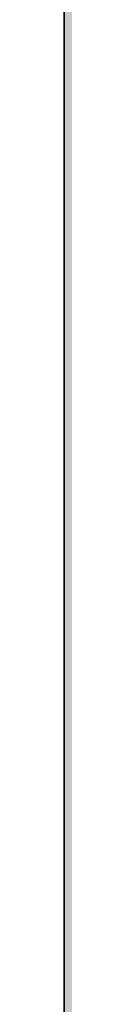
# Model space of a CAD drawing. Units: inches. Extents: x 2091 to 2899, y 967 to 2217.
# Tile 77 of 256: x 2203 to 2203, y 1114 to 1131. Entities that reach past the tile are written whole.
import ezdxf

# ---------------------------------------------------------------- set-up
doc = ezdxf.new("R2010")
doc.units = ezdxf.units.IN
doc.layers.add('A-WALL-PATT', color=141, linetype='Continuous', lineweight=13, true_color=0xadddf7)
doc.layers.add('C-PROP', color=7, linetype='Continuous', lineweight=35)

msp = doc.modelspace()

# ---------------------------------------------------------------- hatches: boundary and pattern name
at = {"layer": 'A-WALL-PATT'}
h = msp.add_hatch(color=256, dxfattribs=at)
h.dxf.hatch_style = 1
h.paths.add_polyline_path([(2212.144, 1941.419), (2387.644, 1941.419), (2387.644, 1824.419), (2392.144, 1824.419), (2392.144, 1941.419), (2609.644, 1941.419), (2609.644, 1825.919), (2614.144, 1825.919), (2614.144, 1941.419), (2794.144, 1941.419), (2794.144, 1928.762), (2803.144, 1928.762), (2803.144, 2050.919), (2203.144, 2050.919), (2203.144, 1900.758), (2212.144, 1900.758)])
h.paths.add_polyline_path([(2212.144, 1945.919), (2212.144, 2041.919), (2794.144, 2041.919), (2794.144, 1945.919), (2402.248, 1945.919), (2401.102, 1945.776), (2398.702, 1945.776)], flags=16)
h.paths.add_polyline_path([(2230.23, 1948.063), (2227.35, 1949.503), (2225.91, 1951.903), (2223.99, 1952.863), (2223.03, 1955.263), (2222.07, 1959.583), (2222.07, 1963.423), (2223.03, 1965.663), (2223.99, 1965.343), (2225.586, 1963.861), (2226.912, 1964.957), (2226.949, 1965.939), (2227.778, 1966.952), (2228.2, 1968.879), (2230.71, 1964.863), (2233.59, 1966.303), (2233.607, 1966.332), (2233.773, 1964.938), (2234.634, 1963.676), (2235.03, 1963.903), (2236.282, 1965.572), (2235.99, 1962.943), (2237.955, 1957.54), (2238.39, 1957.903), (2239.216, 1960.306), (2238.655, 1966.385), (2238.693, 1966.438), (2238.841, 1967.5), (2238.78, 1967.687), (2238.881, 1967.787), (2238.667, 1966.252), (2239.216, 1960.306), (2238.39, 1957.903), (2236.95, 1956.703), (2234.55, 1949.983)], flags=0)
h.paths.add_polyline_path([(2278.012, 1948.063), (2276.496, 1947.873), (2275.85, 1947.689), (2274.652, 1947.103)], flags=0)
h.paths.add_polyline_path([(2269.852, 1955.743), (2268.276, 1956.629), (2270.867, 1956.348), (2269.372, 1958.143), (2268.715, 1959.192), (2270.57, 1958.729), (2268.581, 1961.906), (2270.812, 1960.892), (2270.812, 1963.423), (2271.393, 1964.779), (2270.292, 1966.156), (2271.772, 1965.663), (2272.141, 1966.525), (2273.93, 1965.929), (2275.63, 1968.054), (2276.332, 1966.722), (2276.52, 1966.952), (2276.942, 1968.879), (2277.734, 1967.611), (2278.14, 1969.465), (2279.659, 1967.034), (2280.412, 1966.783), (2280.949, 1967.589), (2281.61, 1967.369), (2282.133, 1968.154), (2282.349, 1966.333), (2282.35, 1966.333), (2283.408, 1968.095), (2283.713, 1965.524), (2284.32, 1964.634), (2284.512, 1964.889), (2284.235, 1965.705), (2284.5, 1967.319), (2284.908, 1965.417), (2285.396, 1966.069), (2285.433, 1966.291), (2285.473, 1966.171), (2286.354, 1967.345), (2286.222, 1966.158), (2287.663, 1968.08), (2287.714, 1968.443), (2288.482, 1969.017), (2288.574, 1968.729), (2288.917, 1969.069), (2288.607, 1966.838), (2288.929, 1963.351), (2288.935, 1963.357), (2288.93, 1963.34), (2289.015, 1962.414), (2290.111, 1963.875), (2290.133, 1963.943), (2290.218, 1964.017), (2290.111, 1963.875), (2289.156, 1960.892), (2288.594, 1959.257), (2288.572, 1959.103), (2289.532, 1960.543), (2290.012, 1962.463), (2290.192, 1962.643), (2289.77, 1959.689), (2286.89, 1957.289), (2284.49, 1950.569), (2283.315, 1950.046), (2283.292, 1949.983), (2280.29, 1948.649), (2281.13, 1948.649), (2282.57, 1948.169), (2283.205, 1948.063), (2278.972, 1948.063), (2276.092, 1949.503), (2274.652, 1951.903), (2272.732, 1952.863)], flags=0)
h.paths.add_polyline_path([(2271.159, 1958.022), (2272.97, 1955.849), (2272.01, 1960.169), (2272.01, 1964.009), (2272.624, 1965.443), (2274.328, 1963.861), (2275.654, 1964.957), (2275.638, 1964.539), (2277.412, 1966.007), (2277.033, 1965.157), (2276.83, 1964.976), (2276.766, 1963.295), (2277.45, 1962.66), (2279.452, 1964.863), (2282.332, 1966.303), (2283.53, 1966.889), (2283.295, 1966.771), (2283.913, 1963.885), (2284.899, 1964.448), (2284.732, 1962.943), (2286.697, 1957.54), (2287.132, 1957.903), (2287.542, 1959.095), (2287.779, 1958.442), (2285.683, 1956.695), (2285.877, 1959.795), (2284.732, 1962.943), (2284.899, 1964.448), (2283.913, 1963.885), (2284.224, 1962.434), (2283.424, 1963.605), (2281.61, 1962.569), (2281.13, 1960.169), (2282.09, 1956.329), (2283.05, 1952.969), (2282.57, 1950.569), (2280.17, 1948.649), (2279.883, 1948.792), (2278.972, 1948.063), (2278.972, 1949.023), (2278.672, 1949.397), (2277.29, 1950.089), (2275.85, 1952.489), (2273.93, 1953.449), (2272.49, 1954.889), (2271.922, 1954.889), (2271.772, 1955.263)], flags=0)
h.paths.add_polyline_path([(2311.994, 1955.743), (2312.063, 1955.674), (2312.055, 1955.709)], flags=0)
h.paths.add_polyline_path([(2331.956, 1963.952), (2333.396, 1965.392), (2331.077, 1963.357), (2330.999, 1963.112)], flags=0)
h.paths.add_polyline_path([(2310.554, 1954.303), (2307.04, 1956.28), (2310.763, 1955.876), (2312.474, 1953.823), (2313.434, 1951.423), (2315.354, 1950.463), (2316.794, 1948.063), (2317.466, 1947.727), (2319.369, 1947.965), (2317.754, 1949.983), (2317.57, 1950.61), (2316.794, 1951.903), (2314.874, 1952.863), (2313.914, 1955.263), (2311.514, 1958.143), (2309.375, 1961.559), (2311.514, 1960.337), (2311.514, 1961.983), (2310.605, 1963.12), (2311.727, 1962.479), (2312.418, 1964.093), (2312.256, 1964.296), (2313.194, 1963.983), (2313.914, 1965.663), (2314.647, 1965.419), (2315.354, 1966.303), (2316.794, 1967.743), (2316.157, 1966.947), (2317.034, 1965.282), (2317.223, 1965.512), (2317.777, 1968.046), (2318.474, 1966.722), (2318.663, 1966.952), (2319.084, 1968.879), (2321.207, 1965.482), (2322.161, 1966.914), (2322.554, 1966.783), (2322.786, 1967.131), (2322.882, 1966.324), (2323.312, 1965.722), (2323.651, 1965.891), (2324.396, 1967.133), (2324.657, 1964.938), (2324.972, 1964.477), (2325.387, 1967.001), (2325.941, 1964.418), (2327.229, 1966.136), (2327.166, 1965.572), (2328.059, 1966.763), (2328.225, 1966.247), (2329.668, 1967.677), (2329.665, 1967.687), (2329.765, 1967.787), (2329.551, 1966.252), (2330.1, 1960.306), (2329.333, 1958.073), (2329.313, 1957.935), (2329.634, 1958.203), (2330.234, 1959.103), (2330.714, 1961.023), (2331.034, 1961.343), (2330.714, 1959.103), (2329.634, 1958.203), (2329.274, 1957.663), (2327.712, 1956.361), (2325.434, 1949.983), (2324.334, 1949.494), (2323.994, 1948.543), (2319.674, 1946.623), (2316.794, 1948.063), (2315.354, 1950.463), (2313.434, 1951.423)], flags=0)
h.paths.add_polyline_path([(2321.336, 1947.952), (2321.114, 1948.063), (2321.114, 1949.023), (2319.194, 1951.423), (2316.794, 1959.583), (2316.663, 1959.583), (2315.354, 1958.143), (2314.394, 1958.143), (2313.148, 1958.709), (2312.954, 1959.583), (2312.954, 1960.892), (2315.834, 1959.583), (2316.663, 1959.583), (2317.315, 1960.299), (2315.03, 1962.421), (2316.356, 1963.517), (2316.372, 1963.952), (2316.47, 1963.861), (2317.796, 1964.957), (2317.755, 1963.89), (2319.175, 1965.157), (2319.498, 1965.881), (2321.114, 1965.343), (2323.236, 1962.372), (2325.686, 1963.773), (2325.543, 1962.481), (2325.199, 1963.494), (2324.479, 1963.082), (2324.926, 1960.994), (2324.078, 1962.236), (2322.415, 1961.286), (2322.074, 1959.583), (2323.034, 1955.743), (2323.994, 1952.383), (2323.514, 1949.983), (2322.143, 1948.886), (2322.074, 1948.543)], flags=0)
h.paths.add_polyline_path([(2320.207, 1963.337), (2320.154, 1963.423), (2320.394, 1963.543)], flags=0)
h.paths.add_polyline_path([(2353.851, 1965.811), (2354.031, 1965.751), (2354.331, 1966.451), (2354.331, 1966.931)], flags=0)
h.paths.add_polyline_path([(2359.021, 1969.026), (2359.098, 1968.902), (2359.234, 1969.52), (2359.234, 1970)], flags=0)
h.paths.add_polyline_path([(2358.257, 1966.682), (2357.984, 1966.348), (2358.211, 1966.146), (2358.41, 1966.39)], flags=0)
h.paths.add_polyline_path([(2357.768, 1966.059), (2357.732, 1965.105), (2357.751, 1965.121), (2357.77, 1965.607), (2357.77, 1966.058)], flags=0)
h.paths.add_polyline_path([(2359.112, 1965.305), (2359.112, 1964.825), (2359.845, 1966.468), (2359.845, 1966.948)], flags=0)
h.paths.add_polyline_path([(2360.224, 1966.621), (2360.699, 1969.363), (2360.699, 1969.843), (2360.211, 1967.026), (2360.211, 1966.643)], flags=0)
h.paths.add_polyline_path([(2363.451, 1967.891), (2363.451, 1968.371), (2362.491, 1966.931), (2362.656, 1966.699)], flags=0)
h.paths.add_polyline_path([(2364.476, 1966.079), (2365.851, 1968.371), (2365.851, 1968.851), (2364.428, 1966.48)], flags=0)
h.paths.add_polyline_path([(2366.314, 1965.853), (2366.367, 1965.696), (2366.803, 1968.346), (2366.803, 1968.826)], flags=0)
h.paths.add_polyline_path([(2367.165, 1965.804), (2367.291, 1966.931), (2367.291, 1967.411), (2367.103, 1965.72)], flags=0)
h.paths.add_polyline_path([(2370.037, 1959.974), (2371.014, 1963.025), (2371.014, 1963.505), (2370.037, 1960.454)], flags=0)
h.paths.add_polyline_path([(2371.611, 1960.211), (2372.571, 1961.651), (2372.571, 1962.131), (2371.803, 1960.979)], flags=0)
h.paths.add_polyline_path([(2350.874, 1956.005), (2351.931, 1955.891), (2354.491, 1953.331), (2353.851, 1954.931), (2351.451, 1957.811), (2347.936, 1963.426), (2347.936, 1963.906), (2351.451, 1958.291), (2353.705, 1955.585), (2352.891, 1959.251), (2352.891, 1959.731), (2352.891, 1961.925), (2356.731, 1959.731), (2358.454, 1961.627), (2354.811, 1965.011), (2355.031, 1965.286), (2358.691, 1961.887), (2361.531, 1965.011), (2364.376, 1966.433), (2364.524, 1965.187), (2365.454, 1963.824), (2365.881, 1964.068), (2365.371, 1966.451), (2365.371, 1966.931), (2366.811, 1960.211), (2366.811, 1959.731), (2366.389, 1952.981), (2367.771, 1956.851), (2368.641, 1957.576), (2366.811, 1962.611), (2366.811, 1963.091), (2368.775, 1957.688), (2369.211, 1958.051), (2370.002, 1960.352), (2369.475, 1966.053), (2369.513, 1966.106), (2369.514, 1966.111), (2369.475, 1966.533), (2369.513, 1966.586), (2369.615, 1967.313), (2369.183, 1968.659), (2369.183, 1969.139), (2369.601, 1967.835), (2369.701, 1967.934), (2369.718, 1968.055), (2370.145, 1968.374), (2369.779, 1968.011), (2369.701, 1967.454), (2370.468, 1968.214), (2369.675, 1967.266), (2369.514, 1966.111), (2370.037, 1960.454), (2370.037, 1959.974), (2369.442, 1958.243), (2370.651, 1959.251), (2371.046, 1962.018), (2371.131, 1962.131), (2370.651, 1958.771), (2367.771, 1956.371), (2365.371, 1949.651), (2362.079, 1948.188), (2363.451, 1947.731), (2361.051, 1947.731), (2360.091, 1947.731), (2357.104, 1947.357), (2360.091, 1948.211), (2358.171, 1949.171), (2356.731, 1951.571), (2354.811, 1952.531), (2351.931, 1955.411)], flags=0)
h.paths.add_polyline_path([(2361.051, 1948.691), (2359.131, 1951.091), (2356.731, 1959.251), (2355.771, 1959.251), (2352.891, 1960.56), (2352.891, 1961.445), (2355.891, 1959.731), (2356.731, 1959.731), (2356.837, 1959.368), (2361.531, 1964.531), (2363.248, 1965.389), (2364.925, 1963.042), (2362.491, 1961.651), (2362.064, 1959.517), (2362.971, 1955.891), (2363.931, 1952.531), (2363.931, 1952.051), (2363.451, 1949.651), (2361.051, 1947.731)], flags=0)
h.paths.add_polyline_path([(2359.131, 1951.571), (2359.291, 1951.371), (2361.051, 1954.451), (2361.051, 1954.931)], flags=0)
h.paths.add_polyline_path([(2357.22, 1966.546), (2356.793, 1968.815), (2356.793, 1969.295), (2357.22, 1967.026)], flags=0)
h.paths.add_polyline_path([(2361.051, 1954.451), (2361.531, 1958.771), (2361.531, 1959.251), (2361.051, 1954.931)], flags=0)
h.paths.add_polyline_path([(2402.548, 1948.486), (2402.302, 1948.416), (2402.59, 1948.416)], flags=0)
h.paths.add_polyline_path([(2394.142, 1956.096), (2395.685, 1954.553), (2396.72, 1953.971), (2396.062, 1955.616), (2395.241, 1956.601), (2395.879, 1956.442), (2395.102, 1959.936), (2395.102, 1963.776), (2396.062, 1966.016), (2397.022, 1965.696), (2398.618, 1964.214), (2399.944, 1965.31), (2399.981, 1966.292), (2400.811, 1967.305), (2401.232, 1969.232), (2403.538, 1965.543), (2403.942, 1967.389), (2404.702, 1967.136), (2405.46, 1966.075), (2406.622, 1966.656), (2406.64, 1966.685), (2406.805, 1965.291), (2406.926, 1965.115), (2407.342, 1964.976), (2407.874, 1965.774), (2408.169, 1964.398), (2409.315, 1965.925), (2409.217, 1965.051), (2409.445, 1963.131), (2410.306, 1961.87), (2410.702, 1962.096), (2411.442, 1963.082), (2411.165, 1963.898), (2411.616, 1966.64), (2411.725, 1966.791), (2411.873, 1967.853), (2411.813, 1968.041), (2411.913, 1968.14), (2411.699, 1966.605), (2412.248, 1960.659), (2413.225, 1963.71), (2414.378, 1964.721), (2414.513, 1965.693), (2414.453, 1965.881), (2414.553, 1965.98), (2414.378, 1964.721), (2414.52, 1964.846), (2414.365, 1964.631), (2414.339, 1964.445), (2414.888, 1958.499), (2414.062, 1956.096), (2412.622, 1954.896), (2410.171, 1948.033), (2410.017, 1948.084), (2405.902, 1946.256), (2405.902, 1947.216), (2405.204, 1948.089), (2404.222, 1948.416), (2403.262, 1948.416), (2400.382, 1949.856), (2399.662, 1951.056), (2397.982, 1952.736), (2397.022, 1953.216), (2395.685, 1954.553), (2392.657, 1956.257)], flags=0)
h.paths.add_polyline_path([(2409.086, 1964.407), (2409.13, 1964.276), (2409.262, 1964.496)], flags=0)
h.paths.add_polyline_path([(2397.742, 1961.616), (2398.702, 1963.856), (2399.662, 1963.536), (2401.427, 1965.741), (2401.791, 1966.559), (2402.071, 1965.071), (2402.836, 1964.393), (2403.262, 1964.915), (2403.338, 1964.771), (2402.616, 1963.976), (2402.499, 1960.902), (2403.543, 1959.932), (2404.413, 1960.89), (2404.702, 1962.336), (2407.916, 1964.172), (2409.52, 1961.927), (2410.987, 1957.893), (2411.422, 1958.256), (2412.048, 1960.076), (2412.41, 1959.079), (2411.676, 1958.467), (2411.662, 1958.256), (2411.626, 1958.426), (2409.982, 1957.056), (2407.582, 1950.336), (2403.262, 1948.416), (2403.262, 1949.376), (2401.342, 1951.776), (2399.417, 1958.324), (2397.742, 1959.085), (2397.742, 1959.97), (2397.102, 1960.336), (2397.742, 1960.045)], flags=0)
h.paths.add_polyline_path([(2405.902, 1952.976), (2405.95, 1953.408), (2406.017, 1953.176)], flags=0)
h.paths.add_polyline_path([(2449.818, 1967.114), (2449.752, 1967.136), (2449.794, 1967.078)], flags=0)
h.paths.add_polyline_path([(2451.698, 1966.618), (2451.741, 1966.69), (2451.692, 1966.666)], flags=0)
h.paths.add_polyline_path([(2454.344, 1965.738), (2455.752, 1967.616), (2455.992, 1968.096), (2454.364, 1965.925)], flags=0)
h.paths.add_polyline_path([(2457.547, 1968.864), (2457.787, 1969.344), (2457.054, 1968.796), (2457.008, 1968.46)], flags=0)
h.paths.add_polyline_path([(2456.922, 1967.857), (2456.802, 1968.229), (2456.723, 1967.66)], flags=0)
h.paths.add_polyline_path([(2457.302, 1967.377), (2457.542, 1967.857), (2456.81, 1966.84), (2456.741, 1966.7), (2456.749, 1966.608)], flags=0)
h.paths.add_polyline_path([(2458.275, 1963.71), (2458.155, 1963.335), (2460.354, 1965.265), (2460.594, 1965.745)], flags=0)
h.paths.add_polyline_path([(2458.392, 1962.816), (2458.364, 1962.618), (2459.592, 1964.256), (2459.832, 1964.736)], flags=0)
h.paths.add_polyline_path([(2459.352, 1962.816), (2459.272, 1962.496), (2460.072, 1963.296), (2460.312, 1963.776)], flags=0)
h.paths.add_polyline_path([(2458.68, 1960.608), (2458.632, 1960.416), (2459.592, 1961.856), (2459.832, 1962.336)], flags=0)
h.paths.add_polyline_path([(2437.838, 1956.243), (2439.192, 1956.096), (2441.352, 1953.936), (2440.872, 1955.136), (2438.472, 1958.016), (2438.072, 1958.656), (2438.712, 1958.496), (2440.64, 1956.183), (2439.912, 1959.456), (2439.912, 1963.296), (2441.352, 1966.656), (2441.592, 1967.136), (2441.112, 1966.016), (2442.072, 1965.696), (2443.989, 1968.092), (2444.241, 1966.751), (2444.917, 1966.152), (2445.677, 1967.08), (2446.255, 1969.725), (2446.495, 1970.205), (2446.282, 1969.232), (2447.363, 1967.503), (2447.72, 1969.568), (2447.96, 1970.048), (2447.485, 1967.307), (2448.792, 1965.216), (2448.472, 1964.864), (2448.552, 1964.736), (2451.452, 1966.186), (2451.615, 1964.811), (2452.308, 1963.796), (2453.235, 1964.326), (2454.072, 1960.416), (2453.629, 1953.318), (2454.792, 1956.576), (2455.032, 1957.056), (2455.719, 1957.628), (2453.832, 1962.816), (2453.941, 1963.794), (2453.335, 1965.578), (2453.824, 1968.551), (2454.064, 1969.031), (2453.575, 1966.058), (2454.04, 1964.688), (2453.832, 1962.816), (2455.719, 1957.628), (2456.367, 1958.168), (2457.058, 1960.179), (2457.298, 1960.659), (2456.472, 1958.256), (2457.718, 1959.294), (2457.672, 1958.976), (2454.89, 1956.657), (2453.614, 1953.085), (2453.592, 1952.736), (2453.352, 1952.256), (2453.36, 1952.372), (2452.632, 1950.336), (2452.392, 1949.856), (2449.204, 1948.439), (2450.712, 1947.936), (2448.072, 1947.936), (2447.112, 1947.936), (2444.552, 1947.616), (2447.2, 1948.372), (2445.192, 1949.376), (2443.752, 1951.776), (2441.832, 1952.736), (2438.952, 1955.616)], flags=0)
h.paths.add_polyline_path([(2443.992, 1959.936), (2444.04, 1959.773), (2444.122, 1959.862)], flags=0)
h.paths.add_polyline_path([(2442.912, 1959.936), (2443.032, 1959.936), (2442.446, 1960.202)], flags=0)
h.paths.add_polyline_path([(2444.983, 1965.02), (2445.279, 1965.265), (2445.519, 1965.745), (2444.994, 1965.31)], flags=0)
h.paths.add_polyline_path([(2446.133, 1965.03), (2446.33, 1965.471), (2444.97, 1964.258), (2444.73, 1963.778)], flags=0)
h.paths.add_polyline_path([(2442.792, 1959.456), (2443.752, 1959.456), (2446.152, 1951.296), (2446.412, 1951.751), (2446.392, 1951.776), (2448.081, 1954.73), (2448.552, 1958.976), (2441.832, 1965.216), (2442.155, 1965.619), (2448.792, 1959.456), (2448.312, 1955.136), (2448.072, 1954.656), (2446.412, 1951.751), (2448.312, 1949.376), (2448.312, 1948.416), (2450.541, 1950.199), (2450.952, 1952.256), (2449.992, 1955.616), (2449.032, 1959.456), (2449.512, 1961.856), (2449.752, 1962.336), (2449.675, 1961.949), (2452.995, 1963.846), (2453.064, 1963.519), (2452.885, 1963.783), (2449.675, 1961.949), (2449.272, 1959.936), (2450.232, 1956.096), (2451.192, 1952.736), (2450.712, 1950.336), (2450.472, 1949.856), (2448.072, 1947.936), (2448.072, 1948.536), (2445.432, 1949.856), (2443.992, 1952.256), (2442.072, 1953.216), (2441.112, 1955.616), (2440.152, 1959.936), (2440.152, 1960.656)], flags=0)
h.paths.add_polyline_path([(2456.692, 1966.986), (2457.608, 1968.081), (2457.848, 1968.561), (2456.932, 1967.466)], flags=0)
h.paths.add_polyline_path([(2489.897, 1966.58), (2489.943, 1966.189), (2490.747, 1967.53), (2491.319, 1968.951)], flags=0)
h.paths.add_polyline_path([(2473.562, 1956.407), (2477.14, 1956.019), (2476.955, 1956.241), (2475.108, 1957.28), (2476.347, 1956.97), (2475.187, 1958.824), (2476.919, 1958.391), (2475.412, 1960.799), (2477.787, 1959.719), (2477.787, 1962.25), (2477.637, 1962.438), (2477.823, 1962.332), (2478.359, 1963.584), (2478.359, 1963.671), (2477.324, 1964.965), (2478.715, 1964.501), (2479.319, 1965.911), (2480.279, 1965.591), (2481.784, 1967.472), (2482.116, 1965.705), (2482.881, 1965.028), (2483.209, 1965.429), (2483.22, 1965.715), (2483.076, 1965.989), (2483.712, 1966.766), (2484.13, 1968.679), (2484.702, 1970.1), (2484.489, 1969.127), (2486.503, 1965.905), (2487.387, 1965.61), (2488.153, 1966.759), (2488.717, 1965.97), (2489.2, 1966.212), (2489.331, 1965.111), (2490.394, 1963.622), (2490.661, 1963.775), (2490.494, 1964.554), (2490.923, 1963.925), (2491.319, 1964.151), (2491.333, 1964.17), (2491.21, 1964.532), (2491.282, 1964.966), (2491.426, 1964.293), (2494.076, 1967.828), (2494.498, 1966.515), (2494.598, 1966.614), (2494.689, 1967.27), (2495.107, 1967.582), (2495.13, 1967.748), (2495.07, 1967.936), (2495.17, 1968.035), (2495.032, 1967.044), (2495.754, 1967.759), (2494.982, 1966.686), (2494.956, 1966.5), (2495.479, 1960.837), (2495.91, 1962.184), (2496.482, 1963.605), (2496.073, 1962.327), (2496.769, 1962.938), (2496.599, 1962.711), (2496.119, 1959.351), (2496.733, 1960.272), (2496.987, 1961.29), (2497.559, 1962.711), (2497.079, 1960.791), (2496.507, 1959.37), (2495.547, 1957.93), (2492.759, 1955.606), (2490.839, 1950.231), (2490.267, 1948.81), (2485.947, 1946.89), (2483.067, 1948.33), (2481.627, 1950.73), (2479.707, 1951.69), (2476.827, 1954.57)], flags=0)
h.paths.add_polyline_path([(2485.577, 1948.313), (2485.559, 1948.311), (2485.579, 1948.311)], flags=0)
h.paths.add_polyline_path([(2478.645, 1954.551), (2478.109, 1956.963), (2479.319, 1955.511), (2480.279, 1953.111), (2482.199, 1952.151), (2483.639, 1949.751), (2486.519, 1948.311), (2486.519, 1949.271), (2484.739, 1951.496), (2484.027, 1950.25), (2481.627, 1958.41), (2482.375, 1959.233), (2482.199, 1959.831), (2483.198, 1960.929), (2479.707, 1964.17), (2480.603, 1965.29), (2481.875, 1964.109), (2482.666, 1964.764), (2482.615, 1963.422), (2482.989, 1963.075), (2484.008, 1963.984), (2484.684, 1965.498), (2484.58, 1965.405), (2485.357, 1967.147), (2485.121, 1965.781), (2486.427, 1963.69), (2488.145, 1964.549), (2489.822, 1962.202), (2490.747, 1962.73), (2492, 1964.4), (2492.076, 1965.087), (2492.213, 1964.684), (2492.485, 1965.047), (2492.279, 1963.191), (2494.244, 1957.788), (2494.563, 1958.054), (2494.933, 1959.133), (2495.505, 1960.554), (2494.679, 1958.151), (2494.107, 1956.73), (2494.563, 1958.054), (2493.409, 1957.092), (2491.707, 1961.77), (2492, 1964.4), (2490.747, 1962.73), (2487.712, 1960.996), (2487.479, 1959.831), (2488.439, 1955.991), (2489.399, 1952.631), (2488.919, 1950.231), (2488.577, 1949.957), (2488.347, 1948.81), (2487.652, 1948.254), (2487.479, 1948.311), (2486.519, 1948.311), (2483.639, 1949.751), (2482.199, 1952.151), (2480.279, 1953.111), (2478.839, 1954.551)], flags=0)
h.paths.add_polyline_path([(2526.648, 1966.988), (2526.517, 1967.031), (2526.6, 1966.915)], flags=0)
h.paths.add_polyline_path([(2528.471, 1966.447), (2528.574, 1966.62), (2528.457, 1966.561)], flags=0)
h.paths.add_polyline_path([(2534.133, 1967.496), (2534.157, 1967.543), (2534.06, 1967.408)], flags=0)
h.paths.add_polyline_path([(2536.162, 1964.051), (2535.157, 1962.711), (2535.101, 1962.316), (2536.117, 1963.671), (2536.421, 1964.278)], flags=0)
h.paths.add_polyline_path([(2535.157, 1959.831), (2536.117, 1961.271), (2536.597, 1962.231), (2535.253, 1960.215)], flags=0)
h.paths.add_polyline_path([(2513.249, 1956.285), (2516.221, 1955.963), (2514.997, 1957.431), (2514.196, 1958.712), (2515.477, 1958.391), (2516.932, 1956.646), (2516.437, 1958.871), (2516.437, 1962.711), (2516.873, 1963.727), (2515.346, 1965.635), (2517.397, 1964.951), (2517.877, 1966.071), (2518.357, 1967.031), (2517.877, 1965.911), (2518.837, 1965.591), (2520.487, 1967.653), (2520.766, 1966.166), (2521.53, 1965.489), (2521.781, 1965.795), (2521.801, 1966.307), (2521.478, 1966.921), (2521.246, 1967.126), (2521.178, 1967.491), (2521.478, 1966.921), (2522.01, 1966.449), (2522.257, 1966.75), (2522.78, 1969.14), (2523.26, 1970.1), (2523.047, 1969.127), (2524.673, 1966.526), (2526.037, 1966.071), (2526.795, 1965.01), (2527.977, 1965.601), (2528.14, 1964.227), (2528.665, 1963.458), (2529.389, 1963.872), (2529.33, 1964.147), (2529.481, 1963.925), (2529.877, 1964.151), (2529.984, 1964.293), (2529.789, 1965.203), (2530.062, 1964.398), (2532.802, 1968.051), (2533.148, 1966.976), (2533.248, 1967.075), (2533.339, 1967.731), (2533.673, 1967.98), (2533.728, 1968.035), (2533.514, 1966.5), (2534.025, 1960.972), (2534.56, 1962.645), (2535.04, 1963.605), (2534.063, 1960.554), (2533.237, 1958.151), (2534.288, 1959.027), (2534.197, 1958.391), (2531.513, 1956.154), (2529.397, 1950.231), (2528.917, 1949.271), (2526.449, 1948.174), (2527.477, 1947.831), (2530.357, 1947.351), (2524.597, 1947.351), (2521.717, 1948.791), (2520.277, 1951.191), (2518.357, 1952.151), (2515.477, 1955.031)], flags=0)
h.paths.add_polyline_path([(2523.935, 1967.19), (2523.62, 1966.484), (2523.77, 1966.242)], flags=0)
h.paths.add_polyline_path([(2518.837, 1953.111), (2517.877, 1955.511), (2516.885, 1959.977), (2516.917, 1959.962), (2516.917, 1962.025), (2520.757, 1959.831), (2522.025, 1961.226), (2518.357, 1964.631), (2519.003, 1965.438), (2520.433, 1964.109), (2521.301, 1964.827), (2521.245, 1963.355), (2525.638, 1959.276), (2526.037, 1961.271), (2529.397, 1963.191), (2530.65, 1964.861), (2530.665, 1964.998), (2530.692, 1964.917), (2531.088, 1965.445), (2530.946, 1964.169), (2530.692, 1964.917), (2529.397, 1963.191), (2526.363, 1961.457), (2526.037, 1959.831), (2526.997, 1955.991), (2527.957, 1952.631), (2527.477, 1950.231), (2527.134, 1949.957), (2526.974, 1949.154), (2526.697, 1949.031), (2524.597, 1947.351), (2524.597, 1948.311), (2524.277, 1948.711), (2522.197, 1949.751), (2520.757, 1952.151)], flags=0)
h.paths.add_polyline_path([(2520.277, 1958.871), (2520.853, 1959.505), (2523.157, 1951.671), (2524.614, 1954.22), (2524.597, 1954.071), (2522.677, 1950.711)], flags=0)
h.paths.add_polyline_path([(2559.371, 1966.311), (2559.398, 1966.325), (2559.402, 1966.345)], flags=0)
h.paths.add_polyline_path([(2549.771, 1957.191), (2552.651, 1954.311), (2552.134, 1955.603), (2550.611, 1957.431), (2547.096, 1963.046), (2545.776, 1965.206), (2549.291, 1959.591), (2551.691, 1956.711), (2550.793, 1960.752), (2550.731, 1960.78), (2550.731, 1964.871), (2551.691, 1967.111), (2552.651, 1966.791), (2554.247, 1965.309), (2555.034, 1965.96), (2555.582, 1966.645), (2555.61, 1967.387), (2556.439, 1968.401), (2556.861, 1970.327), (2559.371, 1966.311), (2560.691, 1964.151), (2562.409, 1965.01), (2561.651, 1966.071), (2560.331, 1968.231), (2561.758, 1966.233), (2562.347, 1967.116), (2562.434, 1966.387), (2563.128, 1965.37), (2563.571, 1965.591), (2563.588, 1965.62), (2563.363, 1967.524), (2563.722, 1965.844), (2565.06, 1968.073), (2564.733, 1965.129), (2565.118, 1963.333), (2567.445, 1966.436), (2567.316, 1967.833), (2567.354, 1967.886), (2567.502, 1968.948), (2567.441, 1969.136), (2567.542, 1969.235), (2567.328, 1967.7), (2567.877, 1961.754), (2568.747, 1964.47), (2568.636, 1965.673), (2568.674, 1965.726), (2568.822, 1966.788), (2568.761, 1966.976), (2568.862, 1967.075), (2568.648, 1965.54), (2568.726, 1964.693), (2568.854, 1964.805), (2568.747, 1964.47), (2568.817, 1963.706), (2568.971, 1963.911), (2568.866, 1963.177), (2569.197, 1959.594), (2568.371, 1957.191), (2566.931, 1955.991), (2564.62, 1949.521), (2564.651, 1949.511), (2564.617, 1949.511), (2564.531, 1949.271), (2560.211, 1947.351), (2557.331, 1948.791), (2556.045, 1950.934), (2556.011, 1950.951), (2555.857, 1951.208), (2553.971, 1952.151), (2551.091, 1955.031), (2546.65, 1957.53)], flags=0)
h.paths.add_polyline_path([(2567.026, 1959.33), (2567.035, 1959.305), (2567.051, 1959.351)], flags=0)
h.paths.add_polyline_path([(2551.968, 1962.518), (2553.011, 1964.951), (2553.971, 1964.631), (2555.567, 1963.149), (2556.893, 1964.246), (2556.93, 1965.227), (2557.144, 1965.489), (2556.42, 1966.131), (2556.391, 1966.105), (2556.38, 1966.166), (2556.42, 1966.131), (2556.952, 1966.605), (2557.092, 1966.919), (2557.571, 1966.01), (2557.759, 1966.241), (2557.418, 1964.68), (2556.893, 1964.246), (2556.807, 1961.998), (2560.691, 1958.391), (2560.636, 1957.893), (2560.811, 1957.191), (2561.771, 1953.831), (2561.291, 1951.431), (2559.11, 1949.687), (2559.156, 1949.629), (2563.027, 1951.349), (2562.611, 1949.271), (2560.211, 1947.351), (2560.211, 1948.311), (2559.251, 1949.511), (2558.891, 1949.511), (2558.891, 1949.961), (2558.291, 1950.711), (2558.054, 1951.518), (2556.971, 1952.871), (2555.068, 1959.341), (2552.051, 1961.065), (2552.051, 1962.471)], flags=0)
h.paths.add_polyline_path([(2588.33, 1958.391), (2588.61, 1958.111), (2588.553, 1958.367)], flags=0)
h.paths.add_polyline_path([(2594.745, 1950.493), (2593.958, 1953.172), (2593.13, 1954.551), (2591.21, 1955.511), (2590.25, 1957.911), (2588.309, 1960.24), (2586.177, 1961.209), (2587.85, 1960.791), (2587.253, 1961.744), (2588.441, 1961.065), (2588.441, 1962.656), (2588.422, 1962.665), (2588.441, 1962.711), (2586.914, 1964.62), (2588.877, 1963.728), (2589.29, 1964.692), (2589.29, 1966.071), (2590.25, 1968.311), (2591.21, 1967.991), (2592.806, 1966.509), (2594.132, 1967.606), (2594.169, 1968.587), (2594.999, 1969.601), (2595.42, 1971.527), (2597.93, 1967.511), (2600.81, 1968.951), (2600.827, 1968.98), (2600.993, 1967.587), (2601.854, 1966.325), (2602.107, 1966.47), (2602.236, 1967.255), (2602.357, 1966.693), (2603.502, 1968.221), (2603.21, 1965.591), (2605.175, 1960.188), (2605.507, 1960.465), (2605.026, 1965.673), (2605.064, 1965.726), (2605.212, 1966.788), (2605.152, 1966.976), (2605.252, 1967.075), (2605.343, 1967.731), (2605.953, 1968.187), (2605.875, 1969.033), (2605.913, 1969.086), (2606.061, 1970.148), (2606, 1970.336), (2606.101, 1970.435), (2605.887, 1968.9), (2606.436, 1962.954), (2605.61, 1960.551), (2605.997, 1960.874), (2606.564, 1962.645), (2608.241, 1964.117), (2608.01, 1963.191), (2607.05, 1961.751), (2606.631, 1961.402), (2606.201, 1958.391), (2603.321, 1955.991), (2600.921, 1949.271), (2596.601, 1947.351), (2593.721, 1948.791), (2592.857, 1950.231), (2592.65, 1950.231)], flags=0)
h.paths.add_polyline_path([(2596.601, 1947.351), (2596.601, 1948.311), (2594.681, 1950.711), (2596.155, 1953.29), (2595.53, 1954.071), (2593.199, 1961.996), (2592.651, 1962.505), (2591.78, 1963.003), (2593.283, 1964.246), (2593.32, 1965.227), (2594.15, 1966.241), (2594.571, 1968.167), (2596.183, 1965.589), (2596.951, 1966.435), (2598.041, 1966.071), (2598.799, 1965.01), (2599.961, 1965.591), (2599.979, 1965.62), (2600.144, 1964.227), (2601.005, 1962.965), (2601.401, 1963.191), (2602.653, 1964.861), (2602.361, 1962.231), (2603.793, 1958.295), (2601.978, 1953.212), (2601.946, 1952.709), (2599.469, 1951.608), (2599.001, 1949.271)], flags=0)
h.paths.add_polyline_path([(2597.561, 1958.871), (2597.671, 1959.419), (2597.595, 1958.736)], flags=0)
h.paths.add_polyline_path([(2623.666, 1961.254), (2625.519, 1960.791), (2624.966, 1961.676), (2627.199, 1960.66), (2627.199, 1961.151), (2626.959, 1962.231), (2626.959, 1963.491), (2625.582, 1965.212), (2626.959, 1964.425), (2626.959, 1965.831), (2626.869, 1965.861), (2627.919, 1968.311), (2628.879, 1967.991), (2630.475, 1966.509), (2631.801, 1967.606), (2631.838, 1968.587), (2632.668, 1969.601), (2633.089, 1971.527), (2635.599, 1967.511), (2638.479, 1968.951), (2638.497, 1968.98), (2638.662, 1967.587), (2639.176, 1966.833), (2639.78, 1967.84), (2640.026, 1966.693), (2641.171, 1968.221), (2640.879, 1965.591), (2641.114, 1964.945), (2641.411, 1965.341), (2641.308, 1964.412), (2642.844, 1960.188), (2643.279, 1960.551), (2644.085, 1962.895), (2643.784, 1966.153), (2643.807, 1966.185), (2643.601, 1968.418), (2643.523, 1968.661), (2643.73, 1970.148), (2643.67, 1970.336), (2643.77, 1970.435), (2643.556, 1968.9), (2643.601, 1968.418), (2643.91, 1967.456), (2644.01, 1967.555), (2643.812, 1966.132), (2644.105, 1962.954), (2644.239, 1961.351), (2644.719, 1961.751), (2645.033, 1962.222), (2645.322, 1963.125), (2646.076, 1963.787), (2645.033, 1962.222), (2644.345, 1960.074), (2643.519, 1957.671), (2642.079, 1956.471), (2639.72, 1949.864), (2639.876, 1949.838), (2635.359, 1947.831), (2632.479, 1949.271), (2631.039, 1951.671), (2629.119, 1952.631), (2628.159, 1955.031), (2625.759, 1957.911)], flags=0)
h.paths.add_polyline_path([(2627.816, 1956.574), (2627.374, 1958.566), (2626.376, 1959.763), (2627.199, 1959.351), (2627.374, 1958.566), (2627.919, 1957.911), (2628.879, 1955.511), (2630.799, 1954.551), (2632.239, 1952.151), (2633.315, 1951.613), (2631.039, 1959.351), (2631.498, 1959.856), (2630.799, 1962.231), (2631.45, 1962.947), (2630.715, 1963.629), (2632.041, 1964.726), (2632.078, 1965.707), (2632.292, 1965.969), (2631.705, 1966.489), (2633.136, 1967.766), (2633.329, 1968.647), (2634.675, 1966.494), (2635.208, 1967.081), (2636.799, 1966.551), (2637.676, 1967.867), (2638.994, 1966.022), (2639.705, 1966.429), (2641.119, 1959.831), (2640.93, 1956.806), (2639.439, 1952.631), (2638.227, 1952.093), (2637.759, 1949.751), (2635.359, 1947.831), (2635.359, 1948.791), (2633.439, 1951.191), (2633.315, 1951.613), (2632.239, 1952.151), (2630.799, 1954.551), (2628.879, 1955.511)], flags=0)
h.paths.add_polyline_path([(2637.759, 1953.831), (2637.279, 1955.511), (2636.319, 1959.351), (2636.799, 1961.751), (2639.234, 1963.142), (2637.557, 1965.49), (2638.739, 1966.081), (2638.902, 1964.707), (2639.763, 1963.445), (2636.799, 1961.751), (2636.532, 1960.418), (2637.039, 1958.391), (2637.999, 1955.031)], flags=0)
h.paths.add_polyline_path([(2668.567, 1951.431), (2667.607, 1953.831), (2665.207, 1956.711), (2662.294, 1961.365), (2665.447, 1959.591), (2666.647, 1958.391), (2666.647, 1959.975), (2666.058, 1960.682), (2666.647, 1960.345), (2666.647, 1961.991), (2666.7, 1962.114), (2666.407, 1963.431), (2666.407, 1967.271), (2667.367, 1969.511), (2668.327, 1969.191), (2669.923, 1967.709), (2671.249, 1968.806), (2671.286, 1969.787), (2672.116, 1970.801), (2672.537, 1972.727), (2675.047, 1968.711), (2677.927, 1970.151), (2677.945, 1970.18), (2678.11, 1968.787), (2678.971, 1967.525), (2679.367, 1967.751), (2680.62, 1969.421), (2680.327, 1966.791), (2682.292, 1961.388), (2682.727, 1961.751), (2683.358, 1963.587), (2683.232, 1964.953), (2683.27, 1965.006), (2683.393, 1965.889), (2683.36, 1966.249), (2683.358, 1966.256), (2683.359, 1966.257), (2682.992, 1970.233), (2683.03, 1970.286), (2683.178, 1971.348), (2683.118, 1971.536), (2683.218, 1971.635), (2683.004, 1970.1), (2683.359, 1966.257), (2683.458, 1966.355), (2683.393, 1965.889), (2683.414, 1965.665), (2684.424, 1966.872), (2683.553, 1964.154), (2683.358, 1963.587), (2683.793, 1958.874), (2682.967, 1956.471), (2681.527, 1955.271), (2680.109, 1951.3), (2680.085, 1950.912), (2679.977, 1950.93), (2679.127, 1948.551), (2674.807, 1946.631), (2671.927, 1948.071), (2670.487, 1950.471)], flags=0)
h.paths.add_polyline_path([(2671.936, 1953.227), (2671.687, 1953.351), (2670.247, 1955.751), (2668.327, 1956.711), (2667.357, 1959.138), (2669.527, 1958.151), (2670.487, 1958.151), (2671.479, 1959.242), (2670.684, 1961.945), (2668.89, 1963.612), (2667.307, 1964.331), (2668.567, 1963.911), (2668.831, 1964.241), (2670.247, 1963.431), (2672.422, 1965.823), (2672.777, 1967.447), (2673.234, 1966.716), (2674.412, 1968.012), (2673.981, 1965.522), (2675.287, 1963.431), (2675.554, 1963.564), (2675.932, 1965.456), (2676.247, 1965.351), (2677.005, 1964.29), (2678.167, 1964.871), (2679.607, 1967.271), (2680.327, 1963.911), (2680.307, 1963.577), (2680.347, 1963.458), (2680.86, 1964.141), (2680.567, 1961.511), (2681.104, 1960.037), (2678.887, 1953.831), (2677.092, 1953.033), (2677.687, 1950.951), (2677.207, 1948.551), (2674.807, 1946.631), (2674.807, 1947.591), (2672.887, 1949.991)], flags=0)
h.paths.add_polyline_path([(2673.985, 1951.911), (2674.567, 1952.931), (2674.567, 1951.911), (2676.967, 1953.831), (2677.447, 1956.231), (2676.487, 1959.591), (2676.247, 1960.551), (2679.73, 1962.541), (2680.059, 1961.002), (2679.211, 1962.245), (2676.247, 1960.551), (2676.487, 1959.591), (2677.447, 1956.231), (2676.967, 1953.831), (2674.567, 1951.911)], flags=0)
h.paths.add_polyline_path([(2707.479, 1952.815), (2706.519, 1955.215), (2705.559, 1959.535), (2705.559, 1963.375), (2706.519, 1965.615), (2707.479, 1965.295), (2709.075, 1963.813), (2710.401, 1964.909), (2710.438, 1965.891), (2711.268, 1966.904), (2711.689, 1968.831), (2714.199, 1964.815), (2717.079, 1966.255), (2717.097, 1966.284), (2717.262, 1964.89), (2718.123, 1963.628), (2718.519, 1963.855), (2719.771, 1965.524), (2719.479, 1962.895), (2721.444, 1957.492), (2721.879, 1957.855), (2722.705, 1960.258), (2722.144, 1966.337), (2722.182, 1966.39), (2722.33, 1967.452), (2722.27, 1967.639), (2722.37, 1967.739), (2722.156, 1966.204), (2722.705, 1960.258), (2721.879, 1957.855), (2720.439, 1956.655), (2718.039, 1949.935), (2713.719, 1948.015), (2710.839, 1949.455), (2709.399, 1951.855)], flags=0)
h.paths.add_polyline_path([(2749.301, 1952.815), (2748.341, 1955.215), (2747.381, 1959.535), (2747.381, 1963.375), (2748.341, 1965.615), (2749.301, 1965.295), (2750.897, 1963.813), (2752.223, 1964.909), (2752.26, 1965.891), (2753.09, 1966.904), (2753.511, 1968.831), (2756.021, 1964.815), (2758.901, 1966.255), (2758.919, 1966.284), (2759.084, 1964.89), (2759.945, 1963.628), (2760.341, 1963.855), (2761.593, 1965.524), (2761.301, 1962.895), (2763.266, 1957.492), (2763.701, 1957.855), (2764.527, 1960.258), (2763.966, 1966.337), (2764.004, 1966.39), (2764.152, 1967.452), (2764.092, 1967.639), (2764.192, 1967.739), (2763.978, 1966.204), (2764.527, 1960.258), (2763.701, 1957.855), (2762.261, 1956.655), (2759.861, 1949.935), (2755.541, 1948.015), (2752.661, 1949.455), (2751.221, 1951.855)], flags=0)
h.paths.add_polyline_path([(2212.144, 1819.935), (2203.144, 1819.935), (2203.144, 1739.98), (2212.144, 1739.98), (2212.144, 1780.919), (2392.144, 1780.919), (2392.144, 1783.919), (2212.144, 1783.919)])
h.paths.add_polyline_path([(2803.144, 1847.939), (2794.144, 1847.939), (2794.144, 1785.419), (2609.644, 1785.419), (2493.876, 1785.419), (2493.876, 1780.919), (2609.644, 1780.919), (2794.144, 1780.919), (2794.144, 1696.919), (2609.376, 1696.919), (2609.376, 1742.919), (2604.876, 1742.919), (2604.876, 1644.419), (2609.376, 1644.419), (2609.376, 1692.419), (2794.144, 1692.419), (2794.144, 1668.165), (2803.144, 1668.165)])
h.paths.add_polyline_path([(2392.144, 1740.419), (2387.644, 1740.419), (2387.644, 1629.419), (2212.144, 1629.419), (2212.144, 1659.156), (2203.144, 1659.156), (2203.144, 1494.089), (2212.144, 1494.089), (2212.144, 1627.919), (2392.144, 1627.919)])
h.paths.add_polyline_path([(2457.876, 1780.919), (2453.376, 1780.919), (2453.376, 1644.419), (2568.876, 1644.419), (2568.876, 1648.919), (2457.876, 1648.919)])
h.paths.add_polyline_path([(2545.144, 1591.919), (2540.644, 1591.919), (2540.644, 1567.919), (2468.644, 1567.919), (2468.644, 1627.919), (2509.144, 1627.919), (2509.144, 1632.419), (2464.144, 1632.419), (2464.144, 1563.419), (2545.144, 1563.419)])
h.paths.add_polyline_path([(2268.644, 1555.919), (2212.144, 1555.919), (2212.144, 1551.419), (2268.644, 1551.419)], flags=17)
h.paths.add_polyline_path([(2212.144, 1413.266), (2203.144, 1413.266), (2203.144, 1233.07), (2212.144, 1233.07)])
h.paths.add_polyline_path([(2267.644, 1351.919), (2212.144, 1351.919), (2212.144, 1347.419), (2267.644, 1347.419)], flags=17)
h.paths.add_polyline_path([(2456.644, 1489.419), (2452.144, 1489.419), (2452.144, 1351.919), (2312.644, 1351.919), (2312.644, 1347.419), (2456.644, 1347.419)])
h.paths.add_polyline_path([(2472.37, 1455.419), (2467.87, 1455.419), (2467.87, 1347.419), (2472.37, 1347.419)])
h.paths.add_polyline_path([(2794.144, 1351.919), (2543.37, 1351.919), (2543.37, 1347.419), (2794.144, 1347.419)], flags=17)
h.paths.add_polyline_path([(2312.644, 1347.419), (2308.144, 1347.419), (2308.144, 1302.162), (2308.342, 1302.164), (2308.144, 1298.169), (2308.144, 1275.419), (2212.144, 1275.419), (2212.144, 1270.919), (2312.644, 1270.919)], flags=17)
h.paths.add_polyline_path([(2212.144, 1152.247), (2203.144, 1152.247), (2203.144, 1090.919), (2803.144, 1090.919), (2803.144, 1392.714), (2794.144, 1392.714), (2794.144, 1143.419), (2548.032, 1143.419), (2548.032, 1138.919), (2794.144, 1138.919), (2794.144, 1099.919), (2212.144, 1099.919)])
h.paths.add_polyline_path([(2471.532, 1266.329, 0.031658), (2467.032, 1269.946), (2467.032, 1143.419), (2471.532, 1143.419), (2471.532, 1148.819)], flags=17)
h.paths.add_polyline_path([(2803.144, 1587.341), (2794.144, 1587.341), (2794.144, 1473.537), (2803.144, 1473.537)])
h.paths.add_polyline_path([(2794.144, 1536.419), (2651.144, 1536.419), (2651.144, 1531.919), (2794.144, 1531.919)])
h.paths.add_polyline_path([(2614.144, 1620.419), (2609.644, 1620.419), (2609.644, 1536.419), (2614.144, 1536.419)])
h.paths.add_polyline_path([(2271.083, 1964.317), (2776.853, 1964.317), (2776.853, 2037.17), (2271.083, 2037.17)], flags=8)
h.paths.add_polyline_path([(2380.649, 1536.824), (2461.041, 1536.824), (2461.041, 1554.653), (2380.649, 1554.653)], flags=9)
h.paths.add_polyline_path([(2203.655, 1608.815), (2316.118, 1608.815), (2316.118, 1621.918), (2203.655, 1621.918)], flags=24)
h.paths.add_polyline_path([(2212.677, 1313.504), (2282.592, 1313.504), (2282.592, 1322.745), (2212.677, 1322.745)], flags=24)
h.paths.add_polyline_path([(2457.112, 1114.779), (2558.482, 1114.779), (2558.482, 1142.22), (2457.112, 1142.22)], flags=25)
h.paths.add_polyline_path([(2473.442, 1273.01), (2604.641, 1273.01), (2604.641, 1318.347), (2473.442, 1318.347)], flags=25)
h.paths.add_polyline_path([(2638.876, 1626.977), (2684.25, 1627.977), (2684.038, 1637.597), (2638.664, 1636.598)], flags=9)
h.paths.add_polyline_path([(2537.591, 1453.793), (2628.39, 1453.793), (2628.39, 1475.345), (2537.591, 1475.345)], flags=9)
h.paths.add_polyline_path([(2504.138, 1714.632), (2554.647, 1714.632), (2554.647, 1730.238), (2504.138, 1730.238)], flags=25)
h.paths.add_polyline_path([(2487.501, 1575.652), (2535.097, 1575.652), (2535.097, 1598.378), (2487.501, 1598.378)], flags=25)
h.paths.add_polyline_path([(2709.099, 1735.71), (2740.017, 1735.71), (2740.017, 1749.938), (2709.099, 1749.938)], flags=25)
h.paths.add_polyline_path([(2442.438, 1792.172), (2564.729, 1792.172), (2564.729, 1842), (2442.438, 1842)], flags=9)
h.paths.add_polyline_path([(2655.816, 1809.644), (2789.52, 1806.694), (2790.085, 1832.292), (2656.381, 1835.242)], flags=25)
h.paths.add_polyline_path([(2234.843, 1797.72), (2368.593, 1794.769), (2369.161, 1820.504), (2235.411, 1823.455)], flags=9)
h.paths.add_polyline_path([(2245.138, 1644.006), (2398.428, 1640.624), (2398.995, 1666.325), (2245.706, 1669.707)], flags=9)
h.paths.add_polyline_path([(2306.143, 1431.169), (2413.768, 1428.794), (2414.333, 1454.392), (2306.708, 1456.766)], flags=9)
h.paths.add_polyline_path([(2306.835, 1458.233), (2393.38, 1456.323), (2393.933, 1481.354), (2307.387, 1483.264)], flags=9)

# ---------------------------------------------------------------- linework, layer by layer
at = {"layer": 'C-PROP'}
msp.add_lwpolyline([(2203.144, 2050.919), (2803.144, 2050.919), (2803.144, 1090.919), (2203.144, 1090.919)], close=True, dxfattribs=at)

doc.saveas('drawing.dxf')
